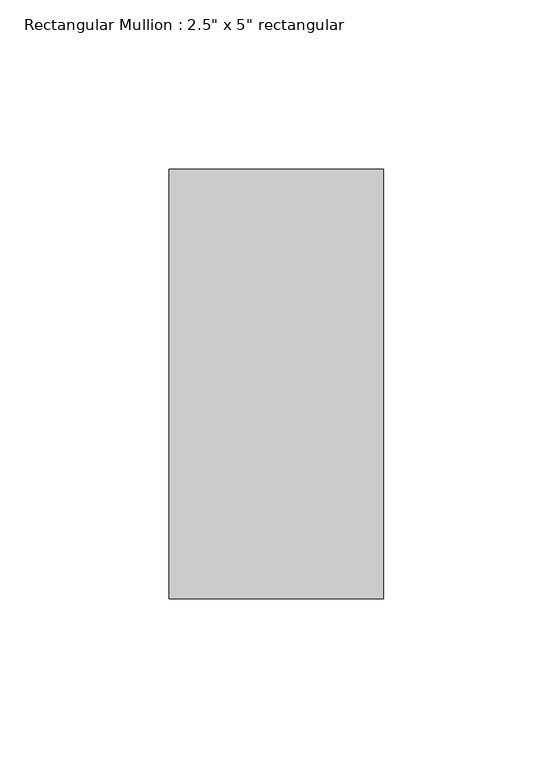
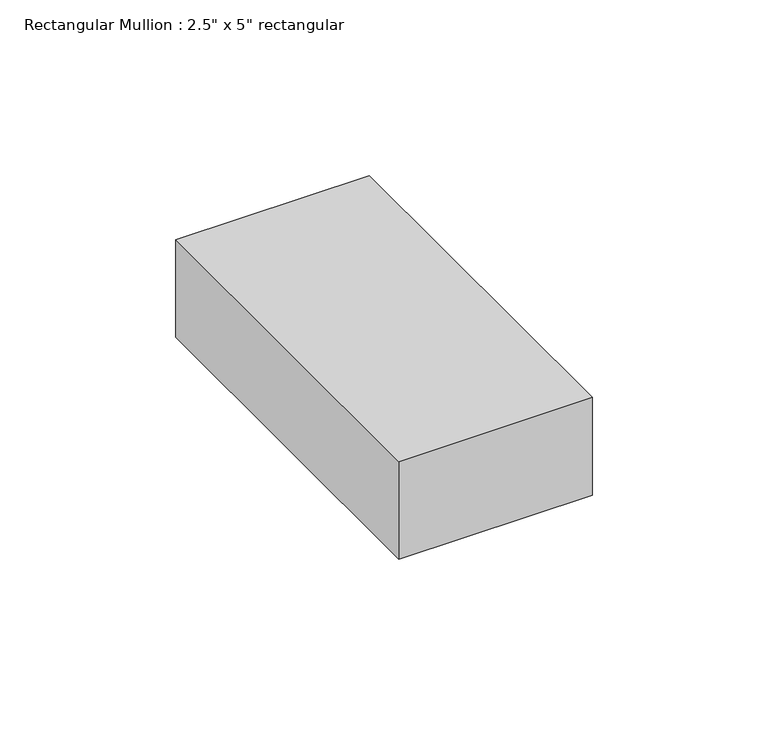
"""IFC4 building model written with IfcOpenShell, lengths in millimetres: member geometry."""

from ifc_helpers import new_model, si_unit, frame, origin, place, context, project, spatial, polyline, outline, extrude, source, transform, mapped, element, save


def member_495a21e7(model_context):
    return source(origin(), model_context, "Body", "SweptSolid", [
        extrude(outline(polyline([(0.0, 63.5), (0.0, -63.5), (-63.5, -63.5), (-63.5, 63.5), (0.0, 63.5)])), frame((0.0, 0.0, -33.8666667), z_axis=(0.0, 0.0, 1.0), x_axis=(1.0, 0.0, 0.0)), (0.0, 0.0, 1.0), 33.8666667),
    ])


if __name__ == "__main__":
    model = new_model("IFC4")
    model_context = context("Model", 3, world=origin())
    ifc_project = project(units=[si_unit("LENGTHUNIT", "METRE", prefix="MILLI")], contexts=[model_context])
    site = spatial("IfcSite", under=ifc_project)
    building = spatial("IfcBuilding", under=site)
    placement = place(None, origin())
    member_shape = member_495a21e7(model_context)
    element("IfcMember", 1, ObjectType="Rectangular Mullion : 2.5\" x 5\" rectangular", at=placement, inside=building, context=model_context, shape_type="MappedRepresentation", body=[
        mapped(member_shape, transform((0.0, 0.0, 0.0), x_axis=(1.0, 0.0, 0.0), y_axis=(0.0, 1.0, 0.0), z_axis=(0.0, 0.0, 1.0))),
    ])
    save(model, "model.ifc")

# Revit data of these elements
# Type "Rectangular Mullion : 2.5\" x 5\" rectangular"
#   built-in parameter 1007304 = 0.416667 (stored number, unit not read)
#   built-in parameter 1007301 = 0.104167 (stored number, unit not read)
#   built-in parameter 1007300 = 0.104167 (stored number, unit not read)
# Element 1 (IfcMember, "Rectangular Mullion : 2.5\" x 5\" rectangular")
#   Materials on its faces: "Aluminum"
# Materials
#   "Aluminum": class "Metal", colour RGB 247 247 247, transparency 0, Description = "Aluminum 6061", Cost = 0
